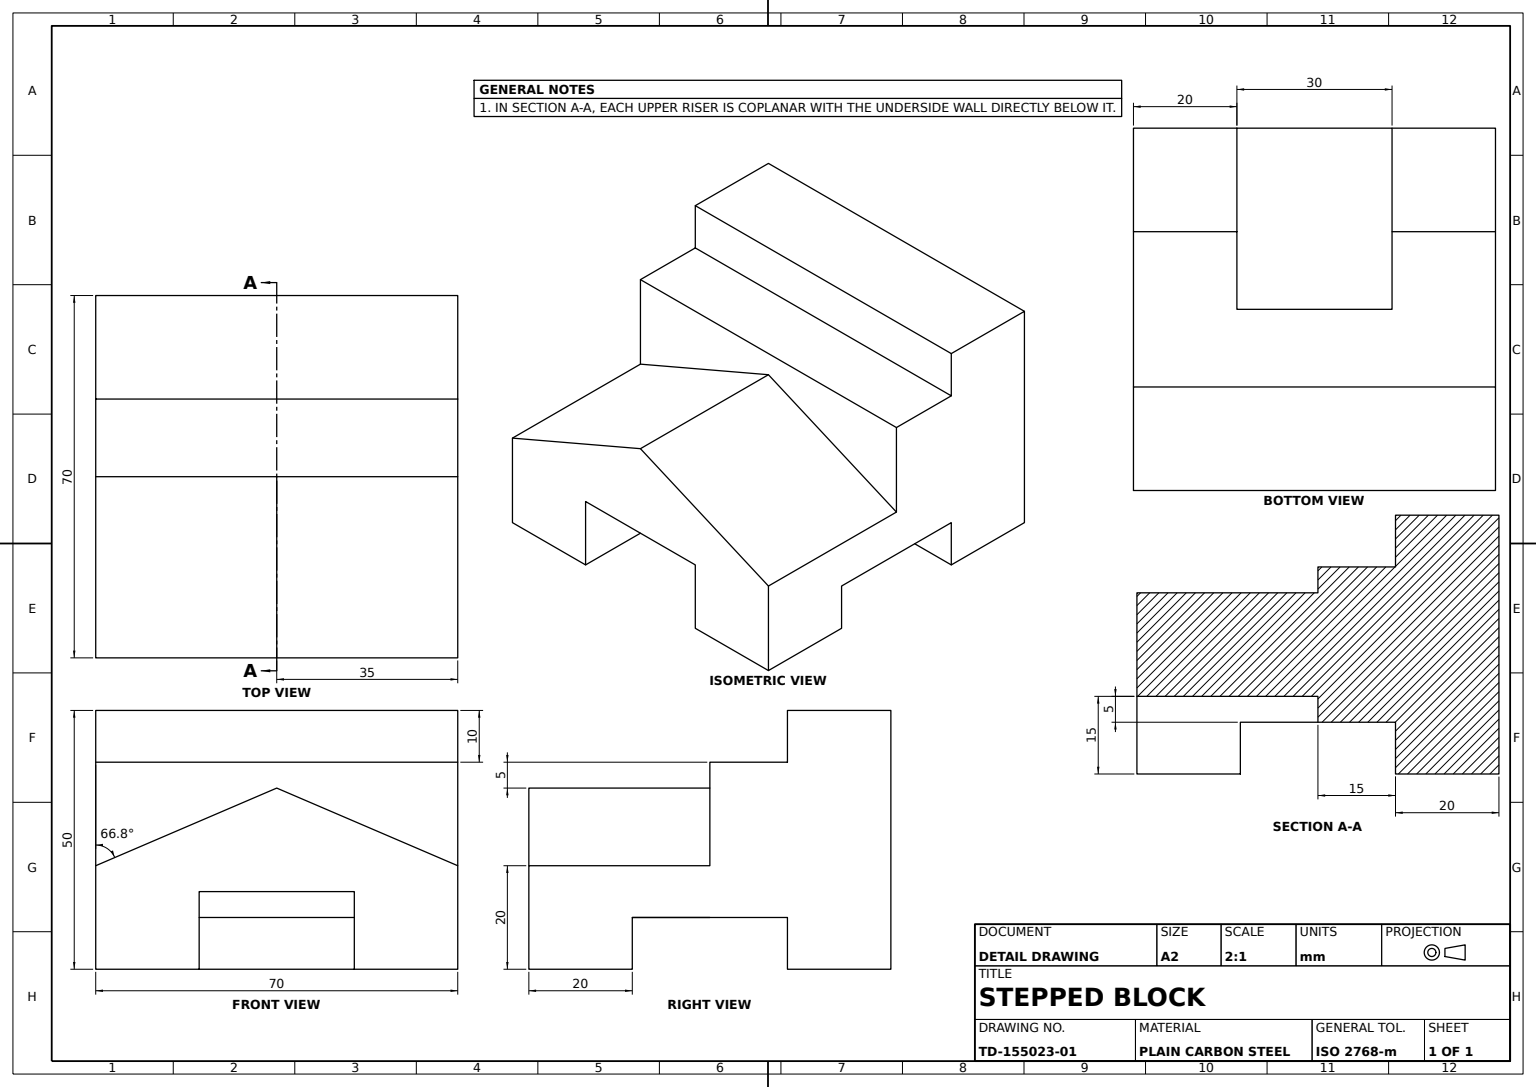
from build123d import *

# Parameters (mm, degrees)
BASE_BLOCK_SKETCH_W  = 70
BASE_BLOCK_SKETCH_H  = 50
BASE_BLOCK_DEPTH     = 15
PAD_SKETCH_W         = 70
PAD_SKETCH_H         = 50
PAD_5MM_DEPTH        = 5
STEPPED_BODY_DEPTH   = 70
ANGLED_WEDGE_DEPTH   = 35
FRONT_SLOT_CUT_DEPTH = 35


with BuildPart() as part:
    # Base Block Sketch → Base Block (new body)
    with BuildSketch(Plane.XY):
        with Locations((35, 25)):
            Rectangle(BASE_BLOCK_SKETCH_W, BASE_BLOCK_SKETCH_H)
    extrude(amount=BASE_BLOCK_DEPTH)

    # Pad Sketch → Pad 5mm (add)
    with BuildSketch(Plane.XY.offset(15)):
        with Locations((35, 25)):
            Rectangle(PAD_SKETCH_W, PAD_SKETCH_H)
    extrude(amount=PAD_5MM_DEPTH)

    # Stepped Profile Sketch → Stepped Body (add)
    with BuildSketch(Plane.ZY):
        Polygon((20, 40), (35, 40), (35, 20), (70, 20), (70, 0), (50, 0), (50, 10), (20, 10), align=None)
    extrude(amount=-STEPPED_BODY_DEPTH)

    # Wedge Sketch → Angled Wedge (add)
    with BuildSketch(Plane.XY.offset(70)):
        Polygon((35, 35), (0, 20), (70, 20), align=None)
    extrude(amount=-ANGLED_WEDGE_DEPTH)

    # Slot Cut Sketch → Front Slot Cut (cut)
    with BuildSketch(Plane.XY.offset(70)):
        Polygon((35, 0), (20, 0), (20, 15), (50, 15), (50, 0), align=None)
    extrude(amount=-FRONT_SLOT_CUT_DEPTH, mode=Mode.SUBTRACT)


solid = part.part
